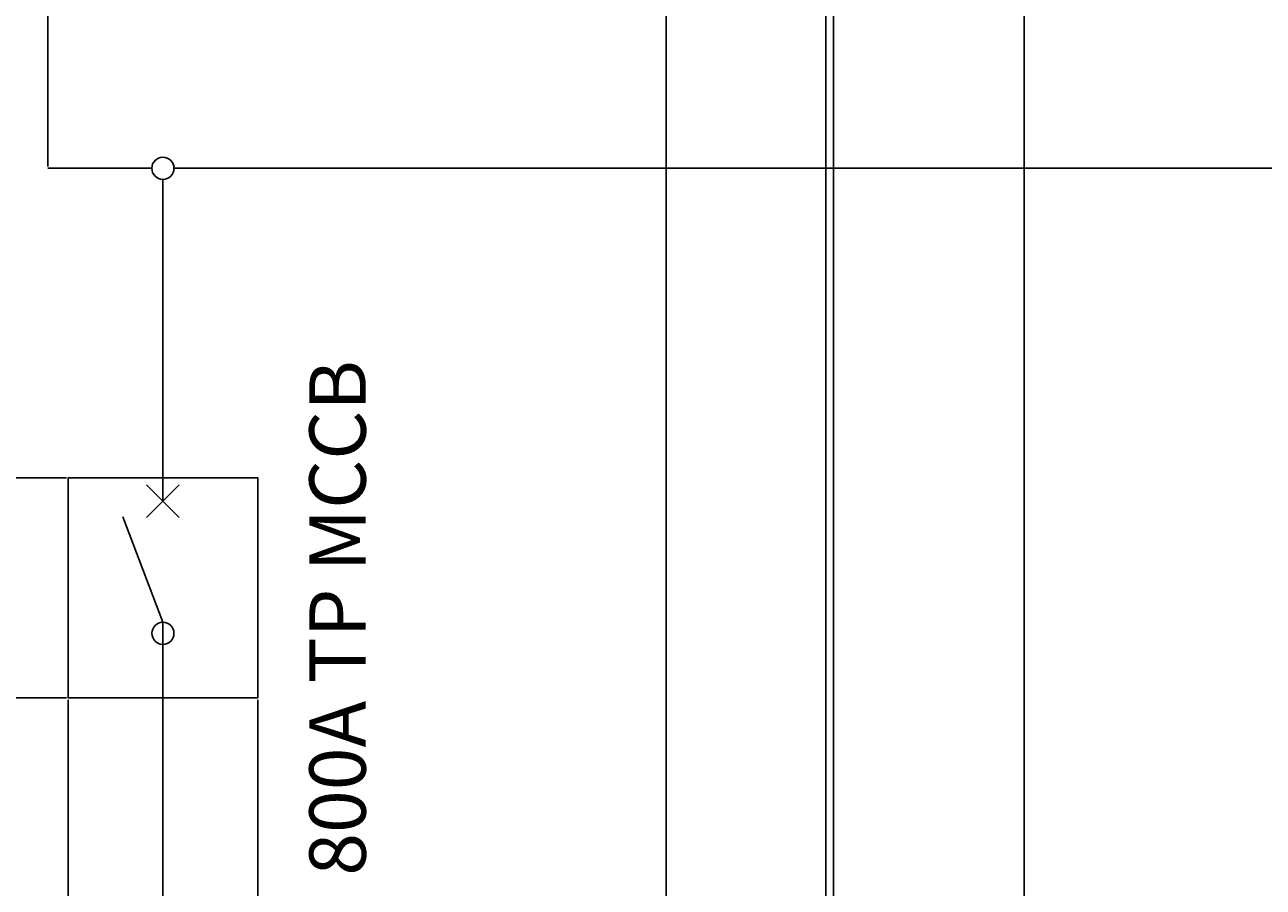
# Model space of a CAD drawing. Units: inches. Extents: x 412 to 584, y 208 to 437.
# Tile 4 of 28: x 450 to 494, y 231 to 262. Entities that reach past the tile are written whole.
import ezdxf

# ---------------------------------------------------------------- set-up
doc = ezdxf.new("R2010")
doc.units = ezdxf.units.IN
doc.header["$MEASUREMENT"] = 0
for name, color, linetype, lineweight in [('A-ANNO-DIMS', 2, 'Continuous', 18), ('E-ANNO-TEXT', 7, 'Continuous', 18), ('E-POWR-EQPM', 3, 'Continuous', 25)]:
    doc.layers.add(name, color=color, linetype=linetype, lineweight=lineweight)
doc.styles.get("Standard").update_dxf_attribs({"font": 'arial.ttf'})
doc.dimstyles.get("Standard").update_dxf_attribs({"dimtxt": 0.18, "dimasz": 0.18, "dimexe": 0.18, "dimexo": 0.0625, "dimgap": 0.09, "dimtad": 0, "dimtih": 1, "dimtoh": 1, "dimdec": 4, "dimzin": 0, "dimdsep": 46, "dimtxsty": 'Standard', "dimcen": 0.09, "dimadec": 0, "dimazin": 0, "dimtfac": 1, "dimtdec": 4, "dimtofl": 0, "dimtmove": 0, "dimatfit": 3, "dimfxl": 1, "dimtolj": 1, "dimtzin": 0, "dimarcsym": 0})

# ---------------------------------------------------------------- blocks, each defined once
blk = doc.blocks.new('*U3')
blk.add_line((-0.212, 0.212), (0.212, -0.212))
blk = doc.blocks.new('*U4')
at = {"color": 0, "linetype": 'ByBlock', "lineweight": -2, "transparency": 16777216}
for p, rotation in [((224.254, 56.203), 180), ((224.677, 56.203), 89.99999999999999), ((224.254, 55.78), 269.9999999999999)]:
    blk.add_blockref('*U3', p, dxfattribs=dict(at, rotation=rotation))
blk.add_blockref('*U3', (224.677, 55.78), dxfattribs=at)
blk = doc.blocks.new('*U7')
blk.add_line((-0.288, 0.288), (0.288, -0.288))
blk = doc.blocks.new('*U8')
at = {"color": 0, "linetype": 'ByBlock', "lineweight": -2, "transparency": 16777216}
for p, rotation in [((224.177, 56.28), 180), ((224.754, 56.28), 90), ((224.177, 55.703), 269.9999999999999)]:
    blk.add_blockref('*U7', p, dxfattribs=dict(at, rotation=rotation))
blk.add_blockref('*U7', (224.754, 55.703), dxfattribs=at)
blk = doc.blocks.new('MCCB-800A')
for q in [(1.94, 18.628), (3.361, 0)]:
    blk.add_line((3.361, 14.893), q)
blk.add_lwpolyline([(0, 20.016), (6.722, 20.016), (6.722, 12.209), (0, 12.209)], close=True)
blk.add_circle((3.361, 14.5), 0.393)
for name in ['*U8', '*U4']:
    blk.add_blockref(name, (-221.104, -36.809))
blk = doc.blocks.new('*D28')
at = {"layer": 'A-ANNO-DIMS', "color": 0, "lineweight": -2, "transparency": 16777216}
for p, q in [((450.562, 256.635), (450.562, 437.465)), ((555.796, 256.635), (555.796, 437.465)), ((450.742, 437.285), (502.724, 437.285)), ((555.616, 437.285), (503.634, 437.285))]:
    blk.add_line(p, q, dxfattribs=at)
at = {"layer": 'A-ANNO-DIMS', "color": 0, "transparency": 16777216}
for points in [[(450.742, 437.315), (450.742, 437.255), (450.562, 437.285)], [(555.616, 437.315), (555.616, 437.255), (555.796, 437.285)]]:
    blk.add_solid(points, dxfattribs=at)
at = {"layer": 'Defpoints', "color": 0, "transparency": 16777216}
for p in [(555.796, 437.285), (450.562, 256.573), (555.796, 256.573)]:
    blk.add_point(p, dxfattribs=at)
at = {"layer": 'A-ANNO-DIMS', "color": 0, "transparency": 16777216, "insert": (503.179, 437.285), "char_height": 0.18, "attachment_point": 5}
blk.add_mtext('\\A1;105.23', dxfattribs=at)
blk = doc.blocks.new('*D33')
at = {"layer": 'A-ANNO-DIMS', "color": 0, "lineweight": -2, "transparency": 16777216}
for p, q in [((472.49, 363.226), (472.49, 208.233)), ((478.422, 363.226), (478.422, 208.233)), ((472.67, 208.413), (475.064, 208.413)), ((478.242, 208.413), (475.849, 208.413))]:
    blk.add_line(p, q, dxfattribs=at)
at = {"layer": 'A-ANNO-DIMS', "color": 0, "transparency": 16777216}
for points in [[(472.67, 208.443), (472.67, 208.383), (472.49, 208.413)], [(478.242, 208.443), (478.242, 208.383), (478.422, 208.413)]]:
    blk.add_solid(points, dxfattribs=at)
at = {"layer": 'Defpoints', "color": 0, "transparency": 16777216}
for p in [(472.49, 363.289), (478.422, 363.289), (478.422, 208.413)]:
    blk.add_point(p, dxfattribs=at)
at = {"layer": 'A-ANNO-DIMS', "color": 0, "transparency": 16777216, "insert": (475.456, 208.413), "char_height": 0.18, "attachment_point": 5}
blk.add_mtext('\\A1;5.932', dxfattribs=at)
blk = doc.blocks.new('*D34')
at = {"layer": 'A-ANNO-DIMS', "color": 0, "lineweight": -2, "transparency": 16777216}
for p, q in [((478.144, 276.254), (478.144, 208.233)), ((485.182, 276.254), (485.182, 208.233)), ((478.324, 208.413), (481.27, 208.413)), ((485.002, 208.413), (482.056, 208.413))]:
    blk.add_line(p, q, dxfattribs=at)
at = {"layer": 'A-ANNO-DIMS', "color": 0, "transparency": 16777216}
for points in [[(478.324, 208.443), (478.324, 208.383), (478.144, 208.413)], [(485.002, 208.443), (485.002, 208.383), (485.182, 208.413)]]:
    blk.add_solid(points, dxfattribs=at)
at = {"layer": 'Defpoints', "color": 0, "transparency": 16777216}
for p in [(478.144, 276.317), (485.182, 276.317), (485.182, 208.413)]:
    blk.add_point(p, dxfattribs=at)
at = {"layer": 'A-ANNO-DIMS', "color": 0, "transparency": 16777216, "insert": (481.663, 208.413), "char_height": 0.18, "attachment_point": 5}
blk.add_mtext('\\A1;7.038', dxfattribs=at)
blk = doc.blocks.new('*D36')
at = {"layer": 'A-ANNO-DIMS', "color": 0, "lineweight": -2, "transparency": 16777216}
for p, q in [((451.283, 237.734), (451.283, 208.233)), ((458.005, 237.734), (458.005, 208.233)), ((451.463, 208.413), (454.251, 208.413)), ((457.825, 208.413), (455.037, 208.413))]:
    blk.add_line(p, q, dxfattribs=at)
at = {"layer": 'A-ANNO-DIMS', "color": 0, "transparency": 16777216}
for points in [[(451.463, 208.443), (451.463, 208.383), (451.283, 208.413)], [(457.825, 208.443), (457.825, 208.383), (458.005, 208.413)]]:
    blk.add_solid(points, dxfattribs=at)
at = {"layer": 'Defpoints', "color": 0, "transparency": 16777216}
for p in [(451.283, 237.797), (458.005, 237.797), (458.005, 208.413)]:
    blk.add_point(p, dxfattribs=at)
at = {"layer": 'A-ANNO-DIMS', "color": 0, "transparency": 16777216, "insert": (454.644, 208.413), "char_height": 0.18, "attachment_point": 5}
blk.add_mtext('\\A1;6.722', dxfattribs=at)
blk = doc.blocks.new('*D37')
at = {"layer": 'A-ANNO-DIMS', "color": 0, "lineweight": -2, "transparency": 16777216}
for p, q in [((451.221, 245.604), (412.276, 245.604)), ((412.456, 245.424), (412.456, 241.882)), ((412.456, 237.977), (412.456, 241.518)), ((451.221, 237.797), (412.276, 237.797))]:
    blk.add_line(p, q, dxfattribs=at)
at = {"layer": 'A-ANNO-DIMS', "color": 0, "transparency": 16777216}
for points in [[(412.426, 245.424), (412.486, 245.424), (412.456, 245.604)], [(412.426, 237.977), (412.486, 237.977), (412.456, 237.797)]]:
    blk.add_solid(points, dxfattribs=at)
at = {"layer": 'Defpoints', "color": 0, "transparency": 16777216}
for p in [(451.283, 245.604), (412.456, 237.797), (451.283, 237.797)]:
    blk.add_point(p, dxfattribs=at)
at = {"layer": 'A-ANNO-DIMS', "color": 0, "transparency": 16777216, "insert": (412.456, 241.7), "char_height": 0.18, "attachment_point": 5}
blk.add_mtext('\\A1;7.807', dxfattribs=at)

msp = doc.modelspace()

# ---------------------------------------------------------------- linework, layer by layer
at = {"layer": 'E-POWR-EQPM'}
for p, q in [((454.2506, 256.5729), (450.562, 256.5729)), ((455.0375, 256.5729), (498.8949, 256.5729)), ((454.6441, 256.1795), (454.6441, 244.7702))]:
    msp.add_line(p, q, dxfattribs=at)
msp.add_circle((454.6441, 256.5729), 0.3935, dxfattribs=at)

# ---------------------------------------------------------------- block references
msp.add_blockref('MCCB-800A', (451.283, 225.588), dxfattribs=at)

# ---------------------------------------------------------------- texts
at = {"layer": 'E-ANNO-TEXT', "insert": (459.8361, 228.1355), "char_height": 2, "attachment_point": 1, "rotation": 90}
msp.add_mtext_dynamic_manual_height_columns('\\pxqc;800A TP MCCB', width=24.999258, gutter_width=1, heights=[6.3954], dxfattribs=at)

# ---------------------------------------------------------------- dimensions: what is measured, and where the dimension line sits
at = {"layer": 'A-ANNO-DIMS'}
for base, p1, p2, override, picture, middle in [((555.7959, 437.2847), (450.562, 256.5729), (555.7959, 256.5729), {"dimdec": 2, "dimlfac": 1, "dimrnd": 0, "dimzin": 0, "dimdsep": 46, "dimlunit": 2}, '*D28', (503.1789, 437.2847)), ((478.4225, 208.4133), (472.4903, 363.2888), (478.4225, 363.2888), {"dimdec": 3, "dimlfac": 1, "dimrnd": 0, "dimzin": 0, "dimdsep": 46, "dimlunit": 2}, '*D33', (475.4564, 208.4133)), ((485.1817, 208.4133), (478.1437, 276.3167), (485.1817, 276.3167), {"dimdec": 3, "dimlfac": 1, "dimrnd": 0, "dimzin": 0, "dimdsep": 46, "dimlunit": 2}, '*D34', (481.6627, 208.4133)), ((458.0051, 208.4133), (451.283, 237.797), (458.0051, 237.797), {"dimdec": 3, "dimlfac": 1, "dimrnd": 0, "dimzin": 0, "dimdsep": 46, "dimlunit": 2}, '*D36', (454.6441, 208.4133))]:
    dim = msp.add_linear_dim(base=base, p1=p1, p2=p2, dimstyle='Standard', override=override, dxfattribs=at)
    dim.commit()
    dim.dimension.update_dxf_attribs({"geometry": picture, "text_midpoint": middle})
dim = msp.add_linear_dim(base=(412.4562, 237.797), p1=(451.283, 245.6036), p2=(451.283, 237.797), angle=90, dimstyle='Standard', override={"dimdec": 3, "dimlfac": 1, "dimrnd": 0, "dimzin": 0, "dimdsep": 46, "dimlunit": 2}, dxfattribs=at)
dim.commit()
dim.dimension.update_dxf_attribs({"geometry": '*D37', "text_midpoint": (412.4562, 241.7003)})

doc.saveas('drawing.dxf')
